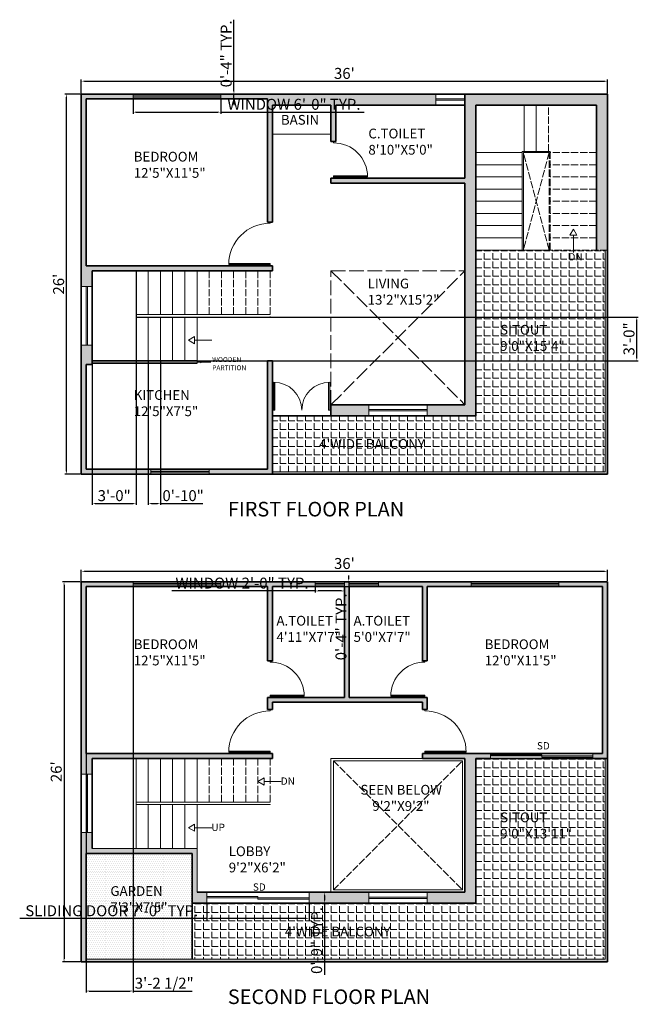
# Model space of a CAD drawing. Units: inches. Extents: x 1947 to 4744, y 610 to 1869.
# Tile 1 of 8: x 1958 to 2466, y 610 to 1419. Entities that reach past the tile are written whole.
import ezdxf

# ---------------------------------------------------------------- set-up
doc = ezdxf.new("R2010")
doc.units = ezdxf.units.IN
doc.linetypes.add('ACAD_ISO02W100', pattern=[15, 12, -3])
for name, color, linetype, lineweight in [('A-ANNO-DIMS', 2, 'Continuous', 18), ('A-ANNO-SYMB', 2, 'Continuous', 18), ('A-ANNO-TEXT', 7, 'Continuous', 18), ('A-ANNO-TITL', 7, 'Continuous', 35), ('A-AREA-IDEN', 7, 'Continuous', 18), ('A-DOOR', 3, 'Continuous', 18), ('A-FLOR-FIXT', 9, 'Continuous', 18), ('A-FLOR-OPEN', 7, 'Continuous', 18), ('A-FLOR-OPEN-PROJ', 8, 'ACAD_ISO02W100', 13), ('A-FLOR-STRS', 7, 'Continuous', 18), ('A-FLOR-STRS-OVHD', 7, 'ACAD_ISO02W100', 13), ('A-GLAZ', 4, 'Continuous', 18), ('A-WALL', 7, 'Continuous', 35), ('A-WALL-PRHT', 7, 'Continuous', 18), ('L-PLNT-PATT', 3, 'Continuous', 13)]:
    doc.layers.add(name, color=color, linetype=linetype, lineweight=lineweight)
doc.layers.add('A-FLOR-PATT', color=251, linetype='Continuous', lineweight=13, true_color=0x636466)
doc.layers.add('A-WALL-PATT', color=18, linetype='Continuous', lineweight=13, true_color=0x000000)
doc.styles.get("Standard").update_dxf_attribs({"font": 'arial.ttf'})
doc.dimstyles.new('ISO-25', dxfattribs={"dimtxt": 9, "dimasz": 2.5, "dimexe": 1.25, "dimexo": 0.625, "dimtad": 1, "dimdec": 1, "dimlunit": 3, "dimtxsty": 'Standard', "dimcen": 2.5, "dimadec": 0, "dimazin": 0, "dimtfac": 1, "dimtdec": 1, "dimtmove": 0, "dimatfit": 3, "dimfxl": 1, "dimarcsym": 0})

# ---------------------------------------------------------------- blocks, each defined once
blk = doc.blocks.new('1')
for p, q in [((4267.36, 1627.82), (4267.36, 1650.82)), ((4268.36, 1627.82), (4268.36, 1650.82)), ((4312.36, 1627.82), (4312.36, 1650.82)), ((4313.36, 1627.82), (4313.36, 1650.82)), ((4266.36, 1627.82), (4268.36, 1627.82)), ((4314.36, 1627.82), (4312.36, 1627.82))]:
    blk.add_line(p, q)
at = {"ltscale": 0.5}
for centre, start, end in [((4267.36, 1627.82), 0, 90), ((4313.36, 1627.82), 90, 180)]:
    blk.add_arc(centre, 23, start, end, dxfattribs=at)
blk = doc.blocks.new('2')
for p, q in [((4319.45, 1679.18), (4319.45, 1713.18)), ((4320.45, 1679.18), (4320.45, 1713.18)), ((4318.45, 1679.18), (4320.45, 1679.18)), ((4353.45, 1679.18), (4354.45, 1679.18))]:
    blk.add_line(p, q)
at = {"ltscale": 0.5}
blk.add_arc((4319.45, 1679.18), 34, 0, 90, dxfattribs=at)
blk = doc.blocks.new('4')
for p, q in [((3808.6, 1693.11), (3808.6, 1721.11)), ((3809.6, 1693.11), (3809.6, 1721.11)), ((3807.6, 1693.11), (3809.6, 1693.11)), ((3836.6, 1693.11), (3837.6, 1693.11))]:
    blk.add_line(p, q)
at = {"ltscale": 0.5}
blk.add_arc((3808.6, 1693.11), 28, 0, 90, dxfattribs=at)
blk = doc.blocks.new('*D66')
at = {"layer": 'A-ANNO-DIMS', "color": 0, "lineweight": -2, "transparency": 16777216}
for p, q in [((2008.18, 1357.67), (1995.32, 1357.67)), ((1996.57, 1048.17), (1996.57, 1355.17)), ((2008.18, 1045.67), (1995.32, 1045.67))]:
    blk.add_line(p, q, dxfattribs=at)
at = {"layer": 'A-ANNO-DIMS', "color": 0, "transparency": 16777216}
for points in [[(1996.15, 1355.17), (1996.99, 1355.17), (1996.57, 1357.67)], [(1996.15, 1048.17), (1996.99, 1048.17), (1996.57, 1045.67)]]:
    blk.add_solid(points, dxfattribs=at)
at = {"layer": 'Defpoints', "color": 0, "transparency": 16777216}
for p in [(1996.57, 1357.67), (2008.81, 1357.67), (2008.81, 1045.67)]:
    blk.add_point(p, dxfattribs=at)
at = {"layer": 'A-ANNO-DIMS', "color": 0, "transparency": 16777216, "insert": (1991.35, 1201.67), "char_height": 9, "attachment_point": 5, "rotation": 90}
blk.add_mtext("26'", dxfattribs=at)
blk = doc.blocks.new('*D67')
at = {"layer": 'A-ANNO-DIMS', "color": 0, "lineweight": -2, "transparency": 16777216}
for p, q in [((2008.81, 1358.29), (2008.81, 1369.55)), ((2011.31, 1368.3), (2438.31, 1368.3)), ((2440.81, 1358.29), (2440.81, 1369.55))]:
    blk.add_line(p, q, dxfattribs=at)
at = {"layer": 'A-ANNO-DIMS', "color": 0, "transparency": 16777216}
for points in [[(2011.31, 1368.71), (2011.31, 1367.88), (2008.81, 1368.3)], [(2438.31, 1368.71), (2438.31, 1367.88), (2440.81, 1368.3)]]:
    blk.add_solid(points, dxfattribs=at)
at = {"layer": 'Defpoints', "color": 0, "transparency": 16777216}
for p in [(2440.81, 1368.3), (2008.81, 1357.67), (2440.81, 1357.67)]:
    blk.add_point(p, dxfattribs=at)
at = {"layer": 'A-ANNO-DIMS', "color": 0, "transparency": 16777216, "insert": (2224.81, 1373.52), "char_height": 9, "attachment_point": 5}
blk.add_mtext("36'", dxfattribs=at)
blk = doc.blocks.new('*D68')
at = {"layer": 'A-ANNO-DIMS', "color": 0, "lineweight": -2, "transparency": 16777216}
for p, q in [((2008.81, 957.97), (2008.81, 967.17)), ((2011.31, 965.92), (2438.31, 965.92)), ((2440.81, 957.97), (2440.81, 967.17))]:
    blk.add_line(p, q, dxfattribs=at)
at = {"layer": 'A-ANNO-DIMS', "color": 0, "transparency": 16777216}
for points in [[(2011.31, 966.33), (2011.31, 965.5), (2008.81, 965.92)], [(2438.31, 966.33), (2438.31, 965.5), (2440.81, 965.92)]]:
    blk.add_solid(points, dxfattribs=at)
at = {"layer": 'Defpoints', "color": 0, "transparency": 16777216}
for p in [(2440.81, 965.92), (2008.81, 957.34), (2440.81, 957.34)]:
    blk.add_point(p, dxfattribs=at)
at = {"layer": 'A-ANNO-DIMS', "color": 0, "transparency": 16777216, "insert": (2224.81, 971.14), "char_height": 9, "attachment_point": 5}
blk.add_mtext("36'", dxfattribs=at)
blk = doc.blocks.new('*D69')
at = {"layer": 'A-ANNO-DIMS', "color": 0, "lineweight": -2, "transparency": 16777216}
for p, q in [((2008.18, 957.34), (1993.38, 957.34)), ((1994.63, 954.84), (1994.63, 647.84)), ((2008.18, 645.34), (1993.38, 645.34))]:
    blk.add_line(p, q, dxfattribs=at)
at = {"layer": 'A-ANNO-DIMS', "color": 0, "transparency": 16777216}
for points in [[(1994.22, 954.84), (1995.05, 954.84), (1994.63, 957.34)], [(1994.22, 647.84), (1995.05, 647.84), (1994.63, 645.34)]]:
    blk.add_solid(points, dxfattribs=at)
at = {"layer": 'Defpoints', "color": 0, "transparency": 16777216}
for p in [(2008.81, 957.34), (1994.63, 645.34), (2008.81, 645.34)]:
    blk.add_point(p, dxfattribs=at)
at = {"layer": 'A-ANNO-DIMS', "color": 0, "transparency": 16777216, "insert": (1989.41, 801.34), "char_height": 9, "attachment_point": 5, "rotation": 90}
blk.add_mtext("26'", dxfattribs=at)
blk = doc.blocks.new('WIN-72-4')
for p, q in [((0, 0), (0, 4)), ((72, 2.5), (0, 2.5)), ((72, 1.5), (0, 1.5)), ((72, 0), (72, 4))]:
    blk.add_line(p, q)
blk = doc.blocks.new('WIN-48-4')
for p, q in [((0, 0), (0, 4)), ((48, 2.5), (0, 2.5)), ((48, 1.5), (0, 1.5)), ((48, 0), (48, 4))]:
    blk.add_line(p, q)
blk = doc.blocks.new('WIN-48-9')
for p, q in [((0, 0), (0, 9)), ((48, 0), (48, 9)), ((48, 5), (0, 5)), ((48, 4), (0, 4))]:
    blk.add_line(p, q)
blk = doc.blocks.new('WIN-24-4')
for p, q in [((0, 0), (0, 4)), ((24, 2.5), (0, 2.5)), ((24, 1.5), (0, 1.5)), ((24, 0), (24, 4))]:
    blk.add_line(p, q)
blk = doc.blocks.new('DOOR-SLIDE-84-9')
for p, q in [((0, 9), (0, 0)), ((84, 9), (84, 0)), ((42, 5.5), (0, 5.5)), ((0, 4.5), (84, 4.5)), ((42, 4.5), (42, 5.5)), ((42, 4.5), (42, 3.5)), ((42, 3.5), (84, 3.5))]:
    blk.add_line(p, q)
blk = doc.blocks.new('DOOR-SLIDE-84-4')
for p, q in [((0, 0), (0, 4)), ((42, 3), (0, 3)), ((0, 2), (84, 2)), ((42, 2), (42, 3)), ((42, 2), (42, 1)), ((42, 1), (84, 1)), ((84, 0), (84, 4))]:
    blk.add_line(p, q)
blk = doc.blocks.new('STAIR-DIRECTION')
blk.add_line((2.91, 14.18), (2.91, 0))
blk.add_lwpolyline([(2.91, 19.23), (0, 14.18), (5.83, 14.18)], close=True)
blk = doc.blocks.new('PARTITION-LEADER')
blk.add_line((3.21, 0.5), (11.48, 0.5))
blk.add_lwpolyline([(0, 0.5), (3.21, 0), (3.21, 0.99)], close=True)
blk = doc.blocks.new('*D86')
at = {"layer": 'A-ANNO-DIMS', "color": 0, "lineweight": -2, "transparency": 16777216}
for p, q in [((2051.31, 1353.04), (2051.31, 1341.62)), ((2123.31, 1353.04), (2123.31, 1341.62)), ((2053.81, 1342.87), (2120.81, 1342.87)), ((2123.31, 1342.87), (2240.95, 1342.87))]:
    blk.add_line(p, q, dxfattribs=at)
at = {"layer": 'A-ANNO-DIMS', "color": 0, "transparency": 16777216}
for points in [[(2053.81, 1343.28), (2053.81, 1342.45), (2051.31, 1342.87)], [(2120.81, 1343.28), (2120.81, 1342.45), (2123.31, 1342.87)]]:
    blk.add_solid(points, dxfattribs=at)
at = {"layer": 'Defpoints', "color": 0, "transparency": 16777216}
for p in [(2051.31, 1353.67), (2123.31, 1353.67), (2123.31, 1342.87)]:
    blk.add_point(p, dxfattribs=at)
at = {"layer": 'A-ANNO-DIMS', "color": 0, "transparency": 16777216, "insert": (2183.38, 1348.15), "char_height": 9, "attachment_point": 5}
blk.add_mtext('WINDOW 6\'-0" TYP.', dxfattribs=at)
blk = doc.blocks.new('*D87')
at = {"layer": 'A-ANNO-DIMS', "color": 0, "lineweight": -2, "transparency": 16777216}
for p, q in [((2134.11, 1360.17), (2134.11, 1418.78)), ((2123.93, 1357.67), (2135.36, 1357.67)), ((2123.93, 1353.67), (2135.36, 1353.67)), ((2134.11, 1353.67), (2134.11, 1357.67)), ((2134.11, 1351.17), (2134.11, 1348.67))]:
    blk.add_line(p, q, dxfattribs=at)
at = {"layer": 'A-ANNO-DIMS', "color": 0, "transparency": 16777216}
for points in [[(2133.69, 1360.17), (2134.52, 1360.17), (2134.11, 1357.67)], [(2133.69, 1351.17), (2134.52, 1351.17), (2134.11, 1353.67)]]:
    blk.add_solid(points, dxfattribs=at)
at = {"layer": 'Defpoints', "color": 0, "transparency": 16777216}
for p in [(2123.31, 1357.67), (2123.31, 1353.67), (2134.11, 1357.67)]:
    blk.add_point(p, dxfattribs=at)
at = {"layer": 'A-ANNO-DIMS', "color": 0, "transparency": 16777216, "insert": (2128.89, 1390.72), "char_height": 9, "attachment_point": 5, "rotation": 90}
blk.add_mtext('0\'-4" TYP.', dxfattribs=at)
blk = doc.blocks.new('*D88')
at = {"layer": 'A-ANNO-DIMS', "color": 0, "lineweight": -2, "transparency": 16777216}
for p, q in [((2200.81, 949.74), (2083.17, 949.74)), ((2200.81, 952.72), (2200.81, 948.49)), ((2222.31, 949.74), (2203.31, 949.74)), ((2224.81, 952.72), (2224.81, 948.49))]:
    blk.add_line(p, q, dxfattribs=at)
at = {"layer": 'A-ANNO-DIMS', "color": 0, "transparency": 16777216}
for points in [[(2203.31, 950.16), (2203.31, 949.33), (2200.81, 949.74)], [(2222.31, 950.16), (2222.31, 949.33), (2224.81, 949.74)]]:
    blk.add_solid(points, dxfattribs=at)
at = {"layer": 'Defpoints', "color": 0, "transparency": 16777216}
for p in [(2200.81, 953.34), (2200.81, 949.74), (2224.81, 953.34)]:
    blk.add_point(p, dxfattribs=at)
at = {"layer": 'A-ANNO-DIMS', "color": 0, "transparency": 16777216, "insert": (2140.74, 955.03), "char_height": 9, "attachment_point": 5}
blk.add_mtext('WINDOW 2\'-0" TYP.', dxfattribs=at)
blk = doc.blocks.new('*D89')
at = {"layer": 'A-ANNO-DIMS', "color": 0, "lineweight": -2, "transparency": 16777216}
for p, q in [((2228.41, 959.84), (2228.41, 962.34)), ((2225.43, 957.34), (2229.66, 957.34)), ((2228.41, 957.34), (2228.41, 953.34)), ((2225.43, 953.34), (2229.66, 953.34)), ((2228.41, 950.84), (2228.41, 892.23))]:
    blk.add_line(p, q, dxfattribs=at)
at = {"layer": 'A-ANNO-DIMS', "color": 0, "transparency": 16777216}
for points in [[(2227.99, 959.84), (2228.82, 959.84), (2228.41, 957.34)], [(2227.99, 950.84), (2228.82, 950.84), (2228.41, 953.34)]]:
    blk.add_solid(points, dxfattribs=at)
at = {"layer": 'Defpoints', "color": 0, "transparency": 16777216}
for p in [(2224.81, 957.34), (2224.81, 953.34), (2228.41, 953.34)]:
    blk.add_point(p, dxfattribs=at)
at = {"layer": 'A-ANNO-DIMS', "color": 0, "transparency": 16777216, "insert": (2223.19, 920.29), "char_height": 9, "attachment_point": 5, "rotation": 90}
blk.add_mtext('0\'-4" TYP.', dxfattribs=at)
blk = doc.blocks.new('*D94')
at = {"layer": 'A-ANNO-DIMS', "color": 0, "lineweight": -2, "transparency": 16777216}
for p, q in [((2111.81, 692.72), (2111.81, 679.49)), ((2195.81, 692.72), (2195.81, 679.49)), ((2111.81, 680.74), (1958.23, 680.74)), ((2193.31, 680.74), (2114.31, 680.74))]:
    blk.add_line(p, q, dxfattribs=at)
at = {"layer": 'A-ANNO-DIMS', "color": 0, "transparency": 16777216}
for points in [[(2114.31, 681.16), (2114.31, 680.33), (2111.81, 680.74)], [(2193.31, 681.16), (2193.31, 680.33), (2195.81, 680.74)]]:
    blk.add_solid(points, dxfattribs=at)
at = {"layer": 'Defpoints', "color": 0, "transparency": 16777216}
for p in [(2111.81, 693.34), (2195.81, 693.34), (2111.81, 680.74)]:
    blk.add_point(p, dxfattribs=at)
at = {"layer": 'A-ANNO-DIMS', "color": 0, "transparency": 16777216, "insert": (2033.77, 686.03), "char_height": 9, "attachment_point": 5}
blk.add_mtext('SLIDING DOOR 7\'-0" TYP.', dxfattribs=at)
blk = doc.blocks.new('*D95')
at = {"layer": 'A-ANNO-DIMS', "color": 0, "lineweight": -2, "transparency": 16777216}
for p, q in [((2196.43, 702.34), (2209.66, 702.34)), ((2208.41, 699.84), (2208.41, 695.84)), ((2196.43, 693.34), (2209.66, 693.34)), ((2208.41, 693.34), (2208.41, 634.73))]:
    blk.add_line(p, q, dxfattribs=at)
at = {"layer": 'A-ANNO-DIMS', "color": 0, "transparency": 16777216}
for points in [[(2207.99, 699.84), (2208.82, 699.84), (2208.41, 702.34)], [(2207.99, 695.84), (2208.82, 695.84), (2208.41, 693.34)]]:
    blk.add_solid(points, dxfattribs=at)
at = {"layer": 'Defpoints', "color": 0, "transparency": 16777216}
for p in [(2195.81, 702.34), (2195.81, 693.34), (2208.41, 693.34)]:
    blk.add_point(p, dxfattribs=at)
at = {"layer": 'A-ANNO-DIMS', "color": 0, "transparency": 16777216, "insert": (2203.19, 662.79), "char_height": 9, "attachment_point": 5, "rotation": 90}
blk.add_mtext('0\'-9" TYP.', dxfattribs=at)
blk = doc.blocks.new('*D101')
at = {"layer": 'A-ANNO-DIMS', "color": 0, "lineweight": -2, "transparency": 16777216}
for p, q in [((2017.81, 1212.04), (2017.81, 1020.37)), ((2053.81, 1212.04), (2053.81, 1020.37)), ((2020.31, 1021.62), (2051.31, 1021.62))]:
    blk.add_line(p, q, dxfattribs=at)
at = {"layer": 'A-ANNO-DIMS', "color": 0, "transparency": 16777216}
for points in [[(2020.31, 1022.03), (2020.31, 1021.2), (2017.81, 1021.62)], [(2051.31, 1022.03), (2051.31, 1021.2), (2053.81, 1021.62)]]:
    blk.add_solid(points, dxfattribs=at)
at = {"layer": 'Defpoints', "color": 0, "transparency": 16777216}
for p in [(2017.81, 1212.67), (2053.81, 1212.67), (2053.81, 1021.62)]:
    blk.add_point(p, dxfattribs=at)
at = {"layer": 'A-ANNO-DIMS', "color": 0, "transparency": 16777216, "insert": (2035.81, 1026.84), "char_height": 9, "attachment_point": 5}
blk.add_mtext('3\'-0"', dxfattribs=at)
blk = doc.blocks.new('*D102')
at = {"layer": 'A-ANNO-DIMS', "color": 0, "lineweight": -2, "transparency": 16777216}
for p, q in [((2054.43, 1174.67), (2466.11, 1174.67)), ((2464.86, 1141.17), (2464.86, 1172.17)), ((2054.43, 1138.67), (2466.11, 1138.67))]:
    blk.add_line(p, q, dxfattribs=at)
at = {"layer": 'A-ANNO-DIMS', "color": 0, "transparency": 16777216}
for points in [[(2464.44, 1172.17), (2465.27, 1172.17), (2464.86, 1174.67)], [(2464.44, 1141.17), (2465.27, 1141.17), (2464.86, 1138.67)]]:
    blk.add_solid(points, dxfattribs=at)
at = {"layer": 'Defpoints', "color": 0, "transparency": 16777216}
for p in [(2053.81, 1174.67), (2464.86, 1174.67), (2053.81, 1138.67)]:
    blk.add_point(p, dxfattribs=at)
at = {"layer": 'A-ANNO-DIMS', "color": 0, "transparency": 16777216, "insert": (2459.63, 1156.67), "char_height": 9, "attachment_point": 5, "rotation": 90}
blk.add_mtext('3\'-0"', dxfattribs=at)
blk = doc.blocks.new('*D103')
at = {"layer": 'A-ANNO-DIMS', "color": 0, "lineweight": -2, "transparency": 16777216}
for p, q in [((2063.81, 1138.04), (2063.81, 1020.37)), ((2073.81, 1138.04), (2073.81, 1020.37)), ((2066.31, 1021.62), (2071.31, 1021.62)), ((2073.81, 1021.62), (2108.47, 1021.62))]:
    blk.add_line(p, q, dxfattribs=at)
at = {"layer": 'A-ANNO-DIMS', "color": 0, "transparency": 16777216}
for points in [[(2066.31, 1022.03), (2066.31, 1021.2), (2063.81, 1021.62)], [(2071.31, 1022.03), (2071.31, 1021.2), (2073.81, 1021.62)]]:
    blk.add_solid(points, dxfattribs=at)
at = {"layer": 'Defpoints', "color": 0, "transparency": 16777216}
for p in [(2063.81, 1138.67), (2073.81, 1138.67), (2073.81, 1021.62)]:
    blk.add_point(p, dxfattribs=at)
at = {"layer": 'A-ANNO-DIMS', "color": 0, "transparency": 16777216, "insert": (2092.39, 1026.84), "char_height": 9, "attachment_point": 5}
blk.add_mtext('0\'-10"', dxfattribs=at)
blk = doc.blocks.new('*D109')
at = {"layer": 'A-ANNO-DIMS', "color": 0, "lineweight": -2, "transparency": 16777216}
for p, q in [((2012.81, 952.72), (2012.81, 620.04)), ((2051.31, 952.72), (2051.31, 620.04)), ((2015.31, 621.29), (2048.81, 621.29)), ((2051.31, 621.29), (2099.95, 621.29))]:
    blk.add_line(p, q, dxfattribs=at)
at = {"layer": 'A-ANNO-DIMS', "color": 0, "transparency": 16777216}
for points in [[(2015.31, 621.71), (2015.31, 620.88), (2012.81, 621.29)], [(2048.81, 621.71), (2048.81, 620.88), (2051.31, 621.29)]]:
    blk.add_solid(points, dxfattribs=at)
at = {"layer": 'Defpoints', "color": 0, "transparency": 16777216}
for p in [(2012.81, 953.34), (2051.31, 953.34), (2051.31, 621.29)]:
    blk.add_point(p, dxfattribs=at)
at = {"layer": 'A-ANNO-DIMS', "color": 0, "transparency": 16777216, "insert": (2076.88, 626.58), "char_height": 9, "attachment_point": 5}
blk.add_mtext('3\'-2 1/2"', dxfattribs=at)

msp = doc.modelspace()

# ---------------------------------------------------------------- hatches: boundary and pattern name
at = {"layer": 'A-FLOR-PATT'}
h = msp.add_hatch(dxfattribs=at)
h.set_pattern_fill('ANGLE', color=256)
h.set_pattern_definition([(0, (-1704.723, -63.1216), (0, 6.985), [5.08, -1.905]), (90, (-1704.723, -63.1216), (-6.985, 4e-16), [5.08, -1.905])])
h.paths.add_polyline_path([(2332.81, 1093.67), (2165.81, 1093.67), (2165.81, 1047.67), (2438.81, 1047.67), (2438.81, 1229.67), (2392.81, 1229.67), (2332.81, 1229.67)])
h.paths.add_polyline_path([(2407.17, 1217.68), (2422.97, 1217.68), (2422.97, 1230.49), (2407.17, 1230.49)], flags=9)
h.paths.add_polyline_path([(2201.93, 1061.9), (2304.85, 1061.9), (2304.85, 1078.98), (2201.93, 1078.98)], flags=24)
h.paths.add_polyline_path([(2349.96, 1142.32), (2406.19, 1142.32), (2406.19, 1172.74), (2349.96, 1172.74)], flags=24)
h = msp.add_hatch(dxfattribs=at)
h.set_pattern_fill('ANGLE', color=256)
h.set_pattern_definition([(0, (-1704.723, -96.523), (0, 6.985), [5.08, -1.905]), (90, (-1704.723, -96.523), (-6.985, 4e-16), [5.08, -1.905])])
h.paths.add_polyline_path([(2438.81, 647.34), (2438.81, 812.34), (2332.81, 812.34), (2332.81, 693.34), (2099.81, 693.34), (2099.81, 647.34)])
h.paths.add_polyline_path([(2173.75, 661.58), (2276.66, 661.58), (2276.66, 678.66), (2173.75, 678.66)], flags=24)
h.paths.add_polyline_path([(2349.96, 742), (2412.1, 742), (2412.1, 772.41), (2349.96, 772.41)], flags=24)
at = {"layer": 'A-WALL-PATT'}
h = msp.add_hatch(color=256, dxfattribs=at)
h.dxf.hatch_style = 1
h.paths.add_polyline_path([(2165.81, 1216.67), (2012.81, 1216.67), (2012.81, 1353.67), (2051.31, 1353.67), (2051.31, 1357.67), (2008.81, 1357.67), (2008.81, 1199.67), (2017.81, 1199.67), (2017.81, 1212.67), (2165.81, 1212.67)])
h.paths.add_polyline_path([(2017.81, 1151.67), (2008.81, 1151.67), (2008.81, 1045.67), (2065.81, 1045.67), (2065.81, 1049.67), (2012.81, 1049.67), (2012.81, 1135.67), (2017.81, 1135.67)])
h.paths.add_polyline_path([(2165.81, 1138.67), (2161.81, 1138.67), (2161.81, 1049.67), (2113.81, 1049.67), (2113.81, 1045.67), (2165.81, 1045.67)])
h.paths.add_polyline_path([(2244.81, 1102.67), (2213.81, 1102.67), (2213.81, 1093.67), (2244.81, 1093.67)])
h.paths.add_polyline_path([(2332.81, 1348.67), (2431.81, 1348.67), (2431.81, 1229.67), (2440.81, 1229.67), (2440.81, 1357.67), (2323.81, 1357.67), (2323.81, 1288.67), (2213.81, 1288.67), (2213.81, 1284.67), (2323.81, 1284.67), (2323.81, 1102.67), (2292.81, 1102.67), (2292.81, 1093.67), (2332.81, 1093.67)])
h.paths.add_polyline_path([(2299.81, 1357.67), (2123.31, 1357.67), (2123.31, 1353.67), (2161.81, 1353.67), (2161.81, 1252.67), (2165.81, 1252.67), (2165.81, 1348.67), (2213.81, 1348.67), (2213.81, 1318.67), (2217.81, 1318.67), (2217.81, 1348.67), (2299.81, 1348.67)])
h.paths.add_polyline_path([(2440.81, 1229.67), (2438.81, 1229.67), (2438.81, 1047.67), (2440.81, 1047.67)])
h.paths.add_polyline_path([(2438.81, 1047.67), (2165.81, 1047.67), (2165.81, 1045.67), (2438.81, 1045.67)])
h.paths.add_polyline_path([(2440.81, 1047.67), (2438.81, 1047.67), (2438.81, 1045.67), (2440.81, 1045.67)])
h = msp.add_hatch(color=256, dxfattribs=at)
h.dxf.hatch_style = 1
h.paths.add_polyline_path([(2228.81, 953.34), (2228.81, 957.34), (2224.81, 957.34), (2224.81, 953.34), (2224.81, 862.34), (2161.81, 862.34), (2161.81, 852.34), (2165.81, 852.34), (2165.81, 858.34), (2288.81, 858.34), (2288.81, 852.34), (2292.81, 852.34), (2292.81, 862.34), (2228.81, 862.34)])
h.paths.add_polyline_path([(2328.81, 957.34), (2252.81, 957.34), (2252.81, 953.34), (2288.81, 953.34), (2288.81, 892.34), (2292.81, 892.34), (2292.81, 953.34), (2328.81, 953.34)])
h.paths.add_polyline_path([(2200.81, 957.34), (2123.31, 957.34), (2123.31, 953.34), (2161.81, 953.34), (2161.81, 892.34), (2165.81, 892.34), (2165.81, 953.34), (2200.81, 953.34)])
h.paths.add_polyline_path([(2440.81, 957.34), (2400.81, 957.34), (2400.81, 953.34), (2436.81, 953.34), (2436.81, 816.34), (2428.81, 816.34), (2428.81, 812.34), (2440.81, 812.34)])
h.paths.add_polyline_path([(2332.81, 812.34), (2344.81, 812.34), (2344.81, 816.34), (2288.81, 816.34), (2288.81, 812.34), (2323.81, 812.34), (2323.81, 702.34), (2292.81, 702.34), (2292.81, 693.34), (2332.81, 693.34)])
h.paths.add_polyline_path([(2244.81, 702.34), (2195.81, 702.34), (2195.81, 693.34), (2244.81, 693.34)], flags=17)
h.paths.add_polyline_path([(2111.81, 702.34), (2103.81, 702.34), (2103.81, 738.34), (2017.81, 738.34), (2017.81, 751.34), (2008.81, 751.34), (2008.81, 645.34), (2012.81, 645.34), (2012.81, 734.34), (2099.81, 734.34), (2099.81, 693.34), (2111.81, 693.34)])
h.paths.add_polyline_path([(2017.81, 812.34), (2165.81, 812.34), (2165.81, 816.34), (2012.81, 816.34), (2012.81, 953.34), (2051.31, 953.34), (2051.31, 957.34), (2008.81, 957.34), (2008.81, 799.34), (2017.81, 799.34)])
h.paths.add_polyline_path([(2440.81, 812.34), (2438.81, 812.34), (2438.81, 647.34), (2012.81, 647.34), (2012.81, 645.34), (2440.81, 645.34)])
at = {"layer": 'L-PLNT-PATT'}
h = msp.add_hatch(dxfattribs=at)
h.set_pattern_fill('DOTS', color=256)
h.set_pattern_definition([(0, (-1704.7231, -102.5354), (0.79375, 1.5875), [0, -1.5875])])
h.paths.add_polyline_path([(2099.81, 647.34), (2099.81, 734.34), (2012.81, 734.34), (2012.81, 647.34)])
h.paths.add_polyline_path([(2030.25, 681.51), (2083.49, 681.51), (2083.49, 711.93), (2030.25, 711.93)], flags=24)

# ---------------------------------------------------------------- linework, layer by layer
at = {"layer": 'A-FLOR-FIXT'}
msp.add_line((2213.81, 1324.67), (2165.81, 1324.67), dxfattribs=at)
at = {"layer": 'A-FLOR-OPEN'}
for points in [[(2323.81, 702.34), (2213.81, 702.34), (2213.81, 812.34), (2323.81, 812.34)], [(2321.81, 704.34), (2215.81, 704.34), (2215.81, 810.34), (2321.81, 810.34)]]:
    msp.add_lwpolyline(points, close=True, dxfattribs=at)
at = {"layer": 'A-FLOR-OPEN-PROJ'}
for p, q in [((2213.81, 1212.67), (2323.81, 1102.67)), ((2213.81, 1102.67), (2323.81, 1212.67))]:
    msp.add_line(p, q, dxfattribs=at)
at = {"layer": 'A-FLOR-OPEN-PROJ', "ltscale": 0.5}
for p, q in [((2215.81, 810.34), (2321.81, 704.34)), ((2215.81, 704.34), (2321.81, 810.34))]:
    msp.add_line(p, q, dxfattribs=at)
at = {"layer": 'A-FLOR-OPEN-PROJ'}
msp.add_lwpolyline([(2323.81, 1102.67), (2213.81, 1102.67), (2213.81, 1212.67), (2323.81, 1212.67)], close=True, dxfattribs=at)
at = {"layer": 'A-FLOR-STRS'}
for p, q in [((2372.31, 1310.67), (2372.31, 1348.67)), ((2382.31, 1310.67), (2382.31, 1348.67)), ((2370.81, 1309.67), (2332.81, 1309.67)), ((2393.81, 1310.67), (2370.81, 1310.67)), ((2370.81, 1229.67), (2370.81, 1310.67)), ((2392.81, 1309.67), (2371.81, 1309.67)), ((2371.81, 1229.67), (2371.81, 1309.67)), ((2370.81, 1299.67), (2332.81, 1299.67)), ((2370.81, 1289.67), (2332.81, 1289.67)), ((2370.81, 1279.67), (2332.81, 1279.67)), ((2370.81, 1269.67), (2332.81, 1269.67)), ((2370.81, 1259.67), (2332.81, 1259.67)), ((2370.81, 1249.67), (2332.81, 1249.67)), ((2370.81, 1239.67), (2332.81, 1239.67)), ((2392.81, 1229.67), (2332.81, 1229.67)), ((2053.81, 1212.67), (2053.81, 1138.67)), ((2063.81, 1212.67), (2063.81, 1176.67)), ((2073.81, 1212.67), (2073.81, 1176.67)), ((2083.81, 1212.67), (2083.81, 1176.67)), ((2093.81, 1212.67), (2093.81, 1176.67)), ((2103.81, 1212.67), (2103.81, 1176.67)), ((2163.81, 1176.67), (2053.81, 1176.67)), ((2053.81, 1174.67), (2163.81, 1174.67)), ((2063.81, 1174.67), (2063.81, 1138.67)), ((2073.81, 1174.67), (2073.81, 1138.67)), ((2083.81, 1174.67), (2083.81, 1138.67)), ((2093.81, 1174.67), (2093.81, 1138.67)), ((2103.81, 1174.67), (2103.81, 1136.67)), ((2053.81, 812.34), (2053.81, 738.34)), ((2063.81, 812.34), (2063.81, 776.34)), ((2073.81, 812.34), (2073.81, 776.34)), ((2083.81, 812.34), (2083.81, 776.34)), ((2093.81, 812.34), (2093.81, 776.34)), ((2103.81, 812.34), (2103.81, 776.34)), ((2163.81, 776.34), (2053.81, 776.34)), ((2053.81, 774.34), (2163.81, 774.34)), ((2063.81, 774.34), (2063.81, 738.34)), ((2073.81, 774.34), (2073.81, 738.34)), ((2083.81, 774.34), (2083.81, 738.34)), ((2093.81, 774.34), (2093.81, 738.34)), ((2103.81, 774.34), (2103.81, 702.34)), ((2017.81, 738.34), (2103.81, 738.34))]:
    msp.add_line(p, q, dxfattribs=at)
at = {"layer": 'A-FLOR-STRS-OVHD', "ltscale": 0.5}
for p, q in [((2392.31, 1310.67), (2392.31, 1348.67)), ((2392.81, 1309.67), (2371.81, 1229.67)), ((2392.81, 1229.67), (2371.81, 1309.67)), ((2392.81, 1229.67), (2392.81, 1309.67)), ((2393.81, 1229.67), (2393.81, 1310.67)), ((2431.81, 1309.67), (2393.81, 1309.67)), ((2431.81, 1299.67), (2393.81, 1299.67)), ((2431.81, 1289.67), (2393.81, 1289.67)), ((2431.81, 1279.67), (2393.81, 1279.67)), ((2431.81, 1269.67), (2393.81, 1269.67)), ((2431.81, 1259.67), (2393.81, 1259.67)), ((2431.81, 1249.67), (2393.81, 1249.67)), ((2431.81, 1239.67), (2393.81, 1239.67)), ((2440.81, 1229.67), (2392.81, 1229.67)), ((2113.81, 1212.67), (2113.81, 1176.67)), ((2123.81, 1212.67), (2123.81, 1176.67)), ((2133.81, 1212.67), (2133.81, 1176.67)), ((2143.81, 1212.67), (2143.81, 1176.67)), ((2153.81, 1212.67), (2153.81, 1176.67)), ((2163.81, 1212.67), (2163.81, 1174.67)), ((2113.81, 812.34), (2113.81, 776.34)), ((2123.81, 812.34), (2123.81, 776.34)), ((2133.81, 812.34), (2133.81, 776.34)), ((2143.81, 812.34), (2143.81, 776.34)), ((2153.81, 812.34), (2153.81, 776.34)), ((2163.81, 812.34), (2163.81, 774.34))]:
    msp.add_line(p, q, dxfattribs=at)
at = {"layer": 'A-GLAZ'}
for p, q in [((2299.81, 1348.67), (2299.81, 1357.67)), ((2323.81, 1353.67), (2299.81, 1353.67)), ((2323.81, 1352.67), (2299.81, 1352.67))]:
    msp.add_line(p, q, dxfattribs=at)
at = {"layer": 'A-WALL'}
for p, q in [((2440.81, 1357.67), (2008.81, 1357.67)), ((2008.81, 1357.67), (2008.81, 1045.67)), ((2161.81, 1353.67), (2012.81, 1353.67)), ((2012.81, 1353.67), (2012.81, 1216.67)), ((2161.81, 1353.67), (2161.81, 1252.67)), ((2323.81, 1288.67), (2323.81, 1357.67)), ((2440.81, 1045.67), (2440.81, 1357.67)), ((2213.81, 1348.67), (2165.81, 1348.67)), ((2165.81, 1348.67), (2165.81, 1252.67)), ((2213.81, 1318.67), (2213.81, 1348.67)), ((2323.81, 1348.67), (2217.81, 1348.67)), ((2217.81, 1318.67), (2217.81, 1348.67)), ((2431.81, 1348.67), (2332.81, 1348.67)), ((2332.81, 1093.67), (2332.81, 1348.67)), ((2431.81, 1229.67), (2431.81, 1348.67)), ((2217.81, 1318.67), (2213.81, 1318.67)), ((2323.81, 1288.67), (2213.81, 1288.67)), ((2213.81, 1284.67), (2213.81, 1288.67)), ((2213.81, 1284.67), (2323.81, 1284.67)), ((2323.81, 1102.67), (2323.81, 1284.67)), ((2165.81, 1252.67), (2161.81, 1252.67)), ((2165.81, 1216.67), (2012.81, 1216.67)), ((2165.81, 1212.67), (2017.81, 1212.67)), ((2017.81, 1212.67), (2017.81, 1135.67)), ((2165.81, 1216.67), (2165.81, 1212.67)), ((2012.81, 1135.67), (2012.81, 1049.67)), ((2012.81, 1135.67), (2017.81, 1135.67)), ((2017.81, 1138.67), (2103.81, 1138.67)), ((2017.81, 1136.67), (2103.81, 1136.67)), ((2161.81, 1138.67), (2165.81, 1138.67)), ((2161.81, 1138.67), (2161.81, 1049.67)), ((2165.81, 1138.67), (2165.81, 1045.67)), ((2213.81, 1102.67), (2213.81, 1093.67)), ((2213.81, 1102.67), (2323.81, 1102.67)), ((2165.81, 1093.67), (2332.81, 1093.67)), ((2008.81, 1045.67), (2440.81, 1045.67)), ((2012.81, 1049.67), (2161.81, 1049.67)), ((2440.81, 957.34), (2008.81, 957.34)), ((2008.81, 957.34), (2008.81, 645.34)), ((2440.81, 645.34), (2440.81, 957.34)), ((2161.81, 953.34), (2012.81, 953.34)), ((2012.81, 953.34), (2012.81, 816.34)), ((2161.81, 953.34), (2161.81, 892.34)), ((2224.81, 953.34), (2165.81, 953.34)), ((2165.81, 953.34), (2165.81, 892.34)), ((2224.81, 862.34), (2224.81, 953.34)), ((2288.81, 953.34), (2228.81, 953.34)), ((2228.81, 862.34), (2228.81, 953.34)), ((2288.81, 892.34), (2288.81, 953.34)), ((2436.81, 953.34), (2292.81, 953.34)), ((2292.81, 892.34), (2292.81, 953.34)), ((2436.81, 816.34), (2436.81, 953.34)), ((2165.81, 892.34), (2161.81, 892.34)), ((2292.81, 892.34), (2288.81, 892.34)), ((2224.81, 862.34), (2161.81, 862.34)), ((2161.81, 862.34), (2161.81, 852.34)), ((2288.81, 858.34), (2165.81, 858.34)), ((2165.81, 858.34), (2165.81, 852.34)), ((2292.81, 862.34), (2228.81, 862.34)), ((2288.81, 852.34), (2288.81, 858.34)), ((2292.81, 852.34), (2292.81, 862.34)), ((2165.81, 852.34), (2161.81, 852.34)), ((2288.81, 852.34), (2292.81, 852.34)), ((2165.81, 816.34), (2012.81, 816.34)), ((2165.81, 812.34), (2017.81, 812.34)), ((2017.81, 812.34), (2017.81, 738.34)), ((2165.81, 816.34), (2165.81, 812.34)), ((2288.81, 816.34), (2436.81, 816.34)), ((2288.81, 812.34), (2288.81, 816.34)), ((2288.81, 812.34), (2323.81, 812.34)), ((2323.81, 702.34), (2323.81, 812.34)), ((2332.81, 693.34), (2332.81, 812.34)), ((2332.81, 812.34), (2440.81, 812.34)), ((2012.81, 734.34), (2012.81, 645.34)), ((2012.81, 734.34), (2099.81, 734.34)), ((2099.81, 734.34), (2099.81, 647.34)), ((2103.81, 702.34), (2323.81, 702.34)), ((2099.81, 693.34), (2332.81, 693.34)), ((2008.81, 645.34), (2440.81, 645.34))]:
    msp.add_line(p, q, dxfattribs=at)
at = {"layer": 'A-WALL-PRHT'}
for p, q in [((2438.81, 1047.67), (2438.81, 1229.67)), ((2165.81, 1047.67), (2438.81, 1047.67)), ((2438.81, 647.34), (2438.81, 812.34)), ((2012.81, 647.34), (2438.81, 647.34))]:
    msp.add_line(p, q, dxfattribs=at)

# ---------------------------------------------------------------- block references
at = {"layer": 'A-ANNO-SYMB'}
msp.add_blockref('STAIR-DIRECTION', (2409.89, 1227.59), dxfattribs=at)
for p, rotation in [((2115.98, 1152.75), 90), ((2173.01, 790.43), 90.00000000000047), ((2115.98, 752.43), 90)]:
    msp.add_blockref('STAIR-DIRECTION', p, dxfattribs=dict(at, rotation=rotation))
at = {"layer": 'A-ANNO-TEXT'}
msp.add_blockref('PARTITION-LEADER', (2103.81, 1137.04), dxfattribs=at)
at = {"layer": 'A-DOOR', "xscale": -1, "rotation": 270}
for name, p in [('4', (522.7, -2518.93)), ('4', (470.7, -2945.26)), ('2', (611.62, -3502.11))]:
    msp.add_blockref(name, p, dxfattribs=at)
at = {"layer": 'A-DOOR'}
for name, p, rotation in [('2', (3842.99, -3101.79), 90.00000000000003), ('4', (3983.92, -2945.26), 90.00000000000003), ('2', (3842.99, -3502.11), 90.00000000000003), ('DOOR-SLIDE-84-4', (2428.81, 816.34), 180), ('DOOR-SLIDE-84-9', (2195.81, 702.34), 180)]:
    msp.add_blockref(name, p, dxfattribs=dict(at, rotation=rotation))
msp.add_blockref('1', (-2100.55, -529.66), dxfattribs=at)
at = {"layer": 'A-GLAZ'}
for name, p in [('WIN-72-4', (2051.31, 1353.67)), ('WIN-48-9', (2244.81, 1093.67)), ('WIN-48-4', (2065.81, 1045.67)), ('WIN-72-4', (2051.31, 953.34)), ('WIN-72-4', (2328.81, 953.34)), ('WIN-48-9', (2244.81, 693.34))]:
    msp.add_blockref(name, p, dxfattribs=at)
for name, p, rotation in [('WIN-48-9', (2008.81, 1199.67), 269.9999999999988), ('WIN-24-4', (2224.81, 957.34), 180), ('WIN-24-4', (2252.81, 957.34), 180), ('WIN-48-9', (2017.81, 751.34), 89.99999999999984)]:
    msp.add_blockref(name, p, dxfattribs=dict(at, rotation=rotation))

# ---------------------------------------------------------------- texts
at = {"layer": 'A-ANNO-TEXT', "attachment_point": 1}
for s, insert, char_height in [('{\\fTimes New Roman|b0|i0|c0|p18;BASIN}', (2172.7, 1340.55), 8), ('{\\fTimes New Roman|b0|i0|c0|p18;DN}', (2408.83, 1227.09), 6), ('{\\fTimes New Roman|b0|i0|c0|p18;WOODEN\\PPARTITION}', (2116.26, 1141.68), 4), ('{\\fTimes New Roman|b0|i0|c0|p18;SD}', (2382.9, 825.67), 6), ('{\\fTimes New Roman|b0|i0|c0|p18;DN}', (2172.59, 796.66), 6), ('{\\fTimes New Roman|b0|i0|c0|p18;UP}', (2115.61, 758.66), 6), ('{\\fTimes New Roman|b0|i0|c0|p18;SD}', (2149.7, 709.67), 6)]:
    msp.add_mtext_dynamic_manual_height_columns(s, width=158.3328, gutter_width=12.5, heights=[0], dxfattribs=dict(at, insert=insert, char_height=char_height))
at = {"layer": 'A-ANNO-TITL', "char_height": 12, "attachment_point": 1}
for s, insert in [('{\\fTimes New Roman|b0|i0|c0|p18;FIRST FLOOR PLAN}', (2129.11, 1022.93)), ('{\\fTimes New Roman|b0|i0|c0|p18;SECOND FLOOR PLAN}', (2129.11, 622.61))]:
    msp.add_mtext_dynamic_manual_height_columns(s, width=253.4596, gutter_width=12.5, heights=[0], dxfattribs=dict(at, insert=insert))
at = {"layer": 'A-AREA-IDEN', "char_height": 8, "attachment_point": 1}
for s, width, heights, insert in [('{\\fTimes New Roman|b0|i0|c0|p18;C.TOILET\\P8\'10"X5\'0"}', 64.3566, [21.47], (2244.5, 1329.31)), ('{\\fTimes New Roman|b0|i0|c0|p18;BEDROOM\\P12\'5"X11\'5"}', 64.3566, [0], (2051.86, 1310.32)), ('{\\fTimes New Roman|b0|i0|c0|p18;LIVING\\P13\'2"X15\'2"}', 64.3566, [21.47], (2243.9, 1206.17)), ('{\\fTimes New Roman|b0|i0|c0|p18;SITOUT\\P9\'0"X15\'4"}', 64.3566, [0], (2352.7, 1168.21)), ('{\\fTimes New Roman|b0|i0|c0|p18;KITCHEN\\P12\'5"X7\'5"}', 64.3566, [0], (2051.86, 1114.62)), ("{\\fTimes New Roman|b0|i0|c0|p18;4'WIDE BALCONY}", 158.3328, [0], (2204.12, 1074.46)), ('{\\fTimes New Roman|b0|i0|c0|p18;A.TOILET\\P4\'11"X7\'7"}', 64.3566, [0], (2169.05, 929.32)), ('{\\fTimes New Roman|b0|i0|c0|p18;A.TOILET\\P5\'0"X7\'7"}', 64.3566, [0], (2232.34, 929.32)), ('{\\fTimes New Roman|b0|i0|c0|p18;BEDROOM\\P12\'5"X11\'5"}', 64.3566, [0], (2051.86, 909.99)), ('{\\fTimes New Roman|b0|i0|c0|p18;BEDROOM\\P12\'0"X11\'5"}', 64.3566, [0], (2340, 909.99)), ('{\\fTimes New Roman|b0|i0|c0|p18;SEEN BELOW\\P    9\'2"X9\'2"}', 135.7043, [0], (2238, 790.55)), ('{\\fTimes New Roman|b0|i0|c0|p18;SITOUT\\P9\'0"X13\'11"}', 64.3566, [0], (2352.7, 767.89)), ('{\\fTimes New Roman|b0|i0|c0|p18;LOBBY\\P9\'2"X6\'2"}', 64.3566, [0], (2129.84, 740.03)), ('{\\fTimes New Roman|b0|i0|c0|p18;GARDEN\\P7\'3"X7\'5"}', 64.3566, [0], (2032.69, 707.4)), ("{\\fTimes New Roman|b0|i0|c0|p18;4'WIDE BALCONY}", 158.3328, [0], (2175.93, 674.13))]:
    msp.add_mtext_dynamic_manual_height_columns(s, width=width, gutter_width=12.5, heights=heights, dxfattribs=dict(at, insert=insert))

# ---------------------------------------------------------------- dimensions: what is measured, and where the dimension line sits
at = {"layer": 'A-ANNO-DIMS'}
for base, p1, p2, angle, text, picture, middle in [((2134.11, 1357.67), (2123.31, 1353.67), (2123.31, 1357.67), 90, '<> TYP.', '*D87', (2128.89, 1390.72)), ((2200.81, 949.74), (2224.81, 953.34), (2200.81, 953.34), 180, 'WINDOW <> TYP.', '*D88', (2140.74, 955.03)), ((2228.41, 953.34), (2224.81, 957.34), (2224.81, 953.34), 270, '<> TYP.', '*D89', (2223.19, 920.29)), ((2111.81, 680.74), (2195.81, 693.34), (2111.81, 693.34), 180, 'SLIDING DOOR <> TYP.', '*D94', (2033.77, 686.03)), ((2208.41, 693.34), (2195.81, 702.34), (2195.81, 693.34), 270, '<> TYP.', '*D95', (2203.19, 662.79))]:
    dim = msp.add_linear_dim(base=base, p1=p1, p2=p2, angle=angle, text=text, dimstyle='ISO-25', override={"dimdec": 1, "dimlfac": 1, "dimrnd": 0, "dimzin": 1, "dimdsep": 46, "dimlunit": 4, "dimfrac": 2}, dxfattribs=at)
    dim.commit()
    dim.dimension.update_dxf_attribs({"geometry": picture, "text_midpoint": middle})
for base, p1, p2, override, picture, middle in [((2440.81, 1368.3), (2008.81, 1357.67), (2440.81, 1357.67), {"dimclrd": 0, "dimclre": 0, "dimclrt": 0}, '*D67', (2224.81, 1373.52)), ((2053.81, 1021.62), (2017.81, 1212.67), (2053.81, 1212.67), {"dimdec": 1, "dimlfac": 1, "dimrnd": 0, "dimzin": 1, "dimdsep": 46, "dimlunit": 4, "dimfrac": 2}, '*D101', (2035.81, 1026.84)), ((2073.81, 1021.62), (2063.81, 1138.67), (2073.81, 1138.67), {"dimdec": 1, "dimlfac": 1, "dimrnd": 0, "dimzin": 1, "dimdsep": 46, "dimlunit": 4, "dimfrac": 2}, '*D103', (2092.39, 1026.84)), ((2440.81, 965.92), (2008.81, 957.34), (2440.81, 957.34), {"dimclrd": 0, "dimclre": 0, "dimclrt": 0}, '*D68', (2224.81, 971.14)), ((2051.31, 621.29), (2012.81, 953.34), (2051.31, 953.34), {"dimdec": 1, "dimlfac": 1, "dimrnd": 0, "dimzin": 1, "dimdsep": 46, "dimlunit": 4, "dimfrac": 2}, '*D109', (2076.88, 626.58))]:
    dim = msp.add_linear_dim(base=base, p1=p1, p2=p2, dimstyle='ISO-25', override=override, dxfattribs=at)
    dim.commit()
    dim.dimension.update_dxf_attribs({"geometry": picture, "text_midpoint": middle})
dim = msp.add_linear_dim(base=(2123.31, 1342.87), p1=(2051.31, 1353.67), p2=(2123.31, 1353.67), text='WINDOW <> TYP.', dimstyle='ISO-25', override={"dimdec": 1, "dimlfac": 1, "dimrnd": 0, "dimzin": 1, "dimdsep": 46, "dimlunit": 4, "dimfrac": 2}, dxfattribs=at)
dim.commit()
dim.dimension.update_dxf_attribs({"geometry": '*D86', "text_midpoint": (2183.38, 1348.15)})
for base, p1, p2, override, picture, middle in [((1996.57, 1357.67), (2008.81, 1045.67), (2008.81, 1357.67), {"dimclrd": 0, "dimclre": 0, "dimclrt": 0}, '*D66', (1991.35, 1201.67)), ((2464.86, 1174.67), (2053.81, 1138.67), (2053.81, 1174.67), {"dimdec": 1, "dimlfac": 1, "dimrnd": 0, "dimzin": 1, "dimdsep": 46, "dimlunit": 4, "dimfrac": 2}, '*D102', (2459.63, 1156.67)), ((1994.63, 645.34), (2008.81, 957.34), (2008.81, 645.34), {"dimclrd": 0, "dimclre": 0, "dimclrt": 0}, '*D69', (1989.41, 801.34))]:
    dim = msp.add_linear_dim(base=base, p1=p1, p2=p2, angle=90, dimstyle='ISO-25', override=override, dxfattribs=at)
    dim.commit()
    dim.dimension.update_dxf_attribs({"geometry": picture, "text_midpoint": middle})

doc.saveas('drawing.dxf')
